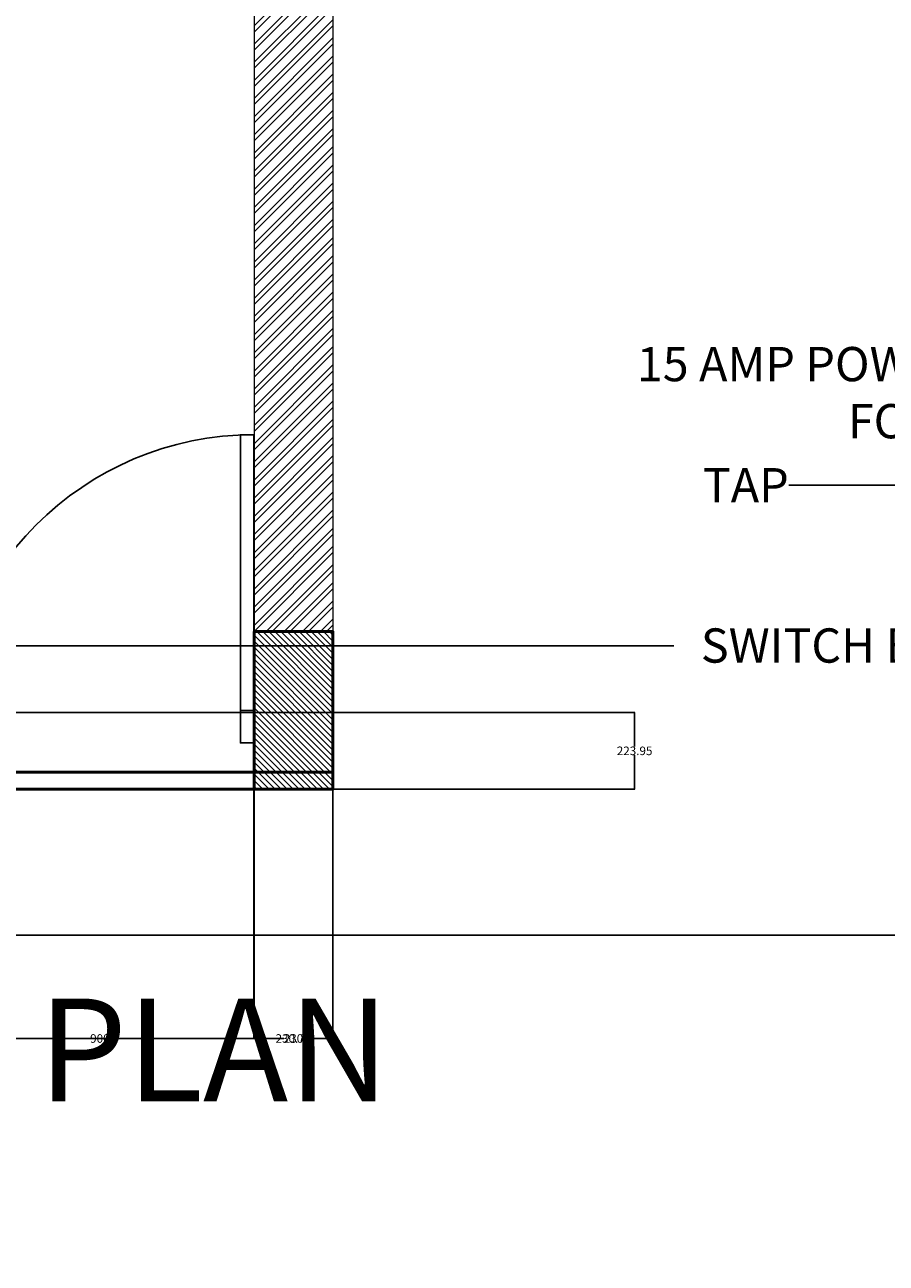
# Model space of a CAD drawing. Units: millimetres. Extents: x 1944 to 29915, y -10550 to 5909.
# Tile 6 of 24: x 9226 to 11743, y -1353 to 2263. Entities that reach past the tile are written whole.
import ezdxf
from ezdxf import colors
from ezdxf.entities.mleader import LeaderData, LeaderLine
from ezdxf.math import Vec2, Vec3

# ---------------------------------------------------------------- set-up
doc = ezdxf.new("R2010")
doc.units = ezdxf.units.MM
doc.header["$MEASUREMENT"] = 0
for name, color, linetype, lineweight in [('A-ANNO-DIMS', 2, 'Continuous', 18), ('A-ANNO-TEXT', 7, 'Continuous', 25), ('A-DOOR', 4, 'Continuous', 25), ('A-FLOR-FIXT', 9, 'Continuous', 18), ('A-WALL', 7, 'Continuous', 50), ('A-WALL-PATT', 8, 'Continuous', 18)]:
    doc.layers.add(name, color=color, linetype=linetype, lineweight=lineweight)
doc.styles.get("Standard").update_dxf_attribs({"font": 'arial.ttf'})
doc.dimstyles.get("Standard").update_dxf_attribs({"dimtxt": 25, "dimasz": 0.18, "dimexe": 0.18, "dimexo": 0.0625, "dimgap": 0.09, "dimtad": 0, "dimtih": 1, "dimtoh": 1, "dimdec": 0, "dimzin": 0, "dimdsep": 46, "dimtxsty": 'Standard', "dimcen": 0.09, "dimadec": 0, "dimazin": 0, "dimtfac": 1, "dimtdec": 0, "dimtofl": 0, "dimtmove": 0, "dimatfit": 3, "dimfxl": 1, "dimtolj": 1, "dimtzin": 0, "dimarcsym": 0})

# ---------------------------------------------------------------- blocks, each defined once
blk = doc.blocks.new('*U2')
for p, q in [((0, 0), (0, -6)), ((40, 0), (40, -6))]:
    blk.add_line(p, q)
blk.add_lwpolyline([(0, 0), (0, 40), (1.75, 40), (1.75, 0)], close=True)
blk.add_arc((0, 0), 40, 0, 90)
blk = doc.blocks.new('*D50')
at = {"layer": 'A-ANNO-DIMS', "color": 0, "lineweight": -2, "transparency": 16777216}
for p, q in [((8995.2, 30.8), (8995.2, -697.2)), ((9895.2, 30.8), (9895.2, -697.2)), ((8995.4, -697), (9417.6, -697)), ((9895, -697), (9472.9, -697))]:
    blk.add_line(p, q, dxfattribs=at)
at = {"layer": 'A-ANNO-DIMS', "color": 0, "transparency": 16777216}
for points in [[(8995.4, -697), (8995.4, -697.1), (8995.2, -697)], [(9895, -697), (9895, -697.1), (9895.2, -697)]]:
    blk.add_solid(points, dxfattribs=at)
at = {"layer": 'Defpoints', "color": 0, "transparency": 16777216}
for p in [(8995.2, 30.8), (9895.2, 30.8), (9895.2, -697)]:
    blk.add_point(p, dxfattribs=at)
at = {"layer": 'A-ANNO-DIMS', "color": 0, "transparency": 16777216, "insert": (9445.2, -697), "char_height": 25, "attachment_point": 5}
blk.add_mtext('\\A1;900', dxfattribs=at)
blk = doc.blocks.new('*D51')
at = {"layer": 'A-ANNO-DIMS', "color": 0, "lineweight": -2, "transparency": 16777216}
for p, q in [((9895.2, 30.8), (9895.2, -697.2)), ((10125.9, 30.8), (10125.9, -697.2)), ((9895.4, -697), (9958.4, -697)), ((10125.8, -697), (10062.8, -697))]:
    blk.add_line(p, q, dxfattribs=at)
at = {"layer": 'A-ANNO-DIMS', "color": 0, "transparency": 16777216}
for points in [[(9895.4, -697), (9895.4, -697.1), (9895.2, -697)], [(10125.8, -697), (10125.8, -697.1), (10125.9, -697)]]:
    blk.add_solid(points, dxfattribs=at)
at = {"layer": 'Defpoints', "color": 0, "transparency": 16777216}
for p in [(9895.2, 30.8), (10125.9, 30.8), (10125.9, -697)]:
    blk.add_point(p, dxfattribs=at)
at = {"layer": 'A-ANNO-DIMS', "color": 0, "transparency": 16777216, "insert": (10010.6, -697), "char_height": 25, "attachment_point": 5}
blk.add_mtext('\\A1;230.73', dxfattribs=at)
blk = doc.blocks.new('*D53')
at = {"layer": 'A-ANNO-DIMS', "color": 0, "lineweight": -2, "transparency": 16777216}
for p, q in [((6945.94205, 490.774608), (6945.94205, -697.212556)), ((9895.94205, 490.774608), (9895.94205, -697.212556)), ((6946.12205, -697.032556), (8383.35205, -697.032556)), ((9895.76205, -697.032556), (8458.53205, -697.032556))]:
    blk.add_line(p, q, dxfattribs=at)
at = {"layer": 'A-ANNO-DIMS', "color": 0, "transparency": 16777216}
for points in [[(6946.12205, -697.002556), (6946.12205, -697.062556), (6945.94205, -697.032556)], [(9895.76205, -697.002556), (9895.76205, -697.062556), (9895.94205, -697.032556)]]:
    blk.add_solid(points, dxfattribs=at)
at = {"layer": 'Defpoints', "color": 0, "transparency": 16777216}
for p in [(6945.94205, 490.837108), (9895.94205, 490.837108), (9895.94205, -697.032556)]:
    blk.add_point(p, dxfattribs=at)
at = {"layer": 'A-ANNO-DIMS', "color": 0, "transparency": 16777216, "insert": (8420.94205, -697.032556), "char_height": 25, "attachment_point": 5}
blk.add_mtext('\\A1;2950', dxfattribs=at)
blk = doc.blocks.new('*D54')
at = {"layer": 'A-ANNO-DIMS', "color": 0, "lineweight": -2, "transparency": 16777216}
for p, q in [((9895.9, 490.8), (9895.9, -697.2)), ((10125.9, 490.8), (10125.9, -697.2)), ((9896.1, -697), (9983.1, -697)), ((10125.8, -697), (10038.8, -697))]:
    blk.add_line(p, q, dxfattribs=at)
at = {"layer": 'A-ANNO-DIMS', "color": 0, "transparency": 16777216}
for points in [[(9896.1, -697), (9896.1, -697.1), (9895.9, -697)], [(10125.8, -697), (10125.8, -697.1), (10125.9, -697)]]:
    blk.add_solid(points, dxfattribs=at)
at = {"layer": 'Defpoints', "color": 0, "transparency": 16777216}
for p in [(9895.9, 490.8), (10125.9, 490.8), (10125.9, -697)]:
    blk.add_point(p, dxfattribs=at)
at = {"layer": 'A-ANNO-DIMS', "color": 0, "transparency": 16777216, "insert": (10010.9, -697), "char_height": 25, "attachment_point": 5}
blk.add_mtext('\\A1;230', dxfattribs=at)
blk = doc.blocks.new('*D56')
at = {"layer": 'A-ANNO-DIMS', "color": 0, "lineweight": -2, "transparency": 16777216}
for p, q in [((8999.7, 254.8), (11007.7, 254.8)), ((11007.5, 254.6), (11007.5, 155.7)), ((11007.5, 31), (11007.5, 130)), ((8995.3, 30.8), (11007.7, 30.8))]:
    blk.add_line(p, q, dxfattribs=at)
at = {"layer": 'A-ANNO-DIMS', "color": 0, "transparency": 16777216}
for points in [[(11007.5, 254.6), (11007.5, 254.6), (11007.5, 254.8)], [(11007.5, 31), (11007.5, 31), (11007.5, 30.8)]]:
    blk.add_solid(points, dxfattribs=at)
at = {"layer": 'Defpoints', "color": 0, "transparency": 16777216}
for p in [(8999.6, 254.8), (8995.2, 30.8), (11007.5, 30.8)]:
    blk.add_point(p, dxfattribs=at)
at = {"layer": 'A-ANNO-DIMS', "color": 0, "transparency": 16777216, "insert": (11007.5, 142.8), "char_height": 25, "attachment_point": 5}
blk.add_mtext('\\A1;223.95', dxfattribs=at)
blk = doc.blocks.new('*D85')
at = {"layer": 'A-ANNO-DIMS', "color": 0, "lineweight": -2, "transparency": 16777216}
for p, q in [((6418.3, -1730.7), (6418.3, -395.6)), ((6418.5, -395.8), (15860.3, -395.8)), ((25389.1, -395.8), (15947.3, -395.8)), ((25389.3, -1846.5), (25389.3, -395.6))]:
    blk.add_line(p, q, dxfattribs=at)
at = {"layer": 'A-ANNO-DIMS', "color": 0, "transparency": 16777216}
for points in [[(6418.5, -395.7), (6418.5, -395.8), (6418.3, -395.8)], [(25389.1, -395.7), (25389.1, -395.8), (25389.3, -395.8)]]:
    blk.add_solid(points, dxfattribs=at)
at = {"layer": 'Defpoints', "color": 0, "transparency": 16777216}
for p in [(25389.3, -395.8), (6418.3, -1730.8), (25389.3, -1846.5)]:
    blk.add_point(p, dxfattribs=at)
at = {"layer": 'A-ANNO-DIMS', "color": 0, "transparency": 16777216, "insert": (15903.8, -395.8), "char_height": 25, "attachment_point": 5}
blk.add_mtext('\\A1;18971', dxfattribs=at)

msp = doc.modelspace()

# ---------------------------------------------------------------- hatches: boundary and pattern name
at = {"layer": 'A-WALL-PATT'}
h = msp.add_hatch(dxfattribs=at)
h.set_pattern_fill('ANSI32', color=256, scale=100)
h.paths.add_polyline_path([(9895.942, 490.837), (10125.942, 490.837), (10125.942, 4760.837), (9895.942, 4760.837)])
h = msp.add_hatch(dxfattribs=at)
h.set_pattern_fill('ANSI31', color=256, scale=100, angle=90)
h.paths.add_polyline_path([(9895.942, 30.837), (10125.942, 30.837), (10125.942, 490.837), (9895.942, 490.837)])

# ---------------------------------------------------------------- linework, layer by layer
at = {"layer": 'A-DOOR'}
msp.add_line((9855.842, 260.837), (9895.942, 260.837), dxfattribs=at)
at = {"layer": 'A-FLOR-FIXT'}
for points in [[(9895.942, 4990.837), (10125.942, 4990.837), (10125.942, 30.837), (9895.217, 30.837)], [(9895.942, 4760.837), (9895.942, 260.837), (9855.842, 260.837)]]:
    msp.add_lwpolyline(points, dxfattribs=at)
at = {"layer": 'A-WALL'}
for p, q in [((10125.942, 81.017), (6715.942, 81.017)), ((10125.942, 30.837), (6715.942, 30.837)), ((8995.217, 30.837), (9895.942, 30.837))]:
    msp.add_line(p, q, dxfattribs=at)
msp.add_lwpolyline([(9895.942, 490.837), (10125.942, 490.837), (10125.942, 30.837), (9895.942, 30.837)], close=True, dxfattribs=at)

# ---------------------------------------------------------------- block references
at = {"layer": 'A-DOOR', "xscale": -22.5, "yscale": 22.5, "zscale": 22.5}
msp.add_blockref('*U2', (9895.217, 165.837), dxfattribs=at)

# ---------------------------------------------------------------- texts
at = {"layer": 'A-ANNO-TEXT'}
msp.add_text('KITCHEN PLAN ', height=300, dxfattribs=at).set_placement((7448.016, -880.236))

# ---------------------------------------------------------------- dimensions: what is measured, and where the dimension line sits
at = {"layer": 'A-ANNO-DIMS'}
for base, p1, p2, override, picture, middle in [((9895.942, -697.033), (6945.942, 490.837), (9895.942, 490.837), {"dimdec": 0, "dimlfac": 1, "dimrnd": 0, "dimzin": 0, "dimdsep": 46, "dimlunit": 2}, '*D53', (8420.942, -697.033)), ((10125.942, -697.033), (9895.942, 490.837), (10125.942, 490.837), {"dimdec": 0, "dimlfac": 1, "dimrnd": 0, "dimzin": 0, "dimdsep": 46, "dimlunit": 2}, '*D54', (10010.942, -697.033)), ((9895.217, -697.033), (8995.217, 30.837), (9895.217, 30.837), {"dimdec": 0, "dimlfac": 1, "dimrnd": 0, "dimzin": 0, "dimdsep": 46, "dimlunit": 2}, '*D50', (9445.217, -697.033)), ((10125.94205, -697.03256), (9895.217, 30.83711), (10125.94205, 30.83711), {"dimdec": 2, "dimlfac": 1, "dimrnd": 0, "dimzin": 0, "dimdsep": 46, "dimlunit": 2}, '*D51', (10010.57953, -697.03256)), ((25389.297, -395.752), (6418.315, -1730.752), (25389.297, -1846.542), {"dimdec": 0, "dimlfac": 1, "dimrnd": 0, "dimzin": 0, "dimdsep": 46, "dimlunit": 2}, '*D85', (15903.806, -395.752))]:
    dim = msp.add_linear_dim(base=base, p1=p1, p2=p2, dimstyle='Standard', override=override, dxfattribs=at)
    dim.commit()
    dim.dimension.update_dxf_attribs({"geometry": picture, "text_midpoint": middle})
dim = msp.add_linear_dim(base=(11007.504, 30.837), p1=(8999.621, 254.791), p2=(8995.217, 30.837), angle=90, dimstyle='Standard', override={"dimdec": 2, "dimlfac": 1, "dimrnd": 0, "dimzin": 0, "dimdsep": 46, "dimlunit": 2}, dxfattribs=at)
dim.commit()
dim.dimension.update_dxf_attribs({"geometry": '*D56', "text_midpoint": (11007.504, 142.814)})

# ---------------------------------------------------------------- leaders
at = {"layer": 'A-ANNO-TEXT'}
ml = msp.add_multileader_mtext('Standard', dxfattribs=at)
ml.set_content('15 AMP POWER POINT \\PFOR GEYSER ', color=256)
ml.set_leader_properties()
ml.build(insert=Vec2(0, 0))
ml.multileader.update_dxf_attribs({"dogleg_length": 0.36, "arrow_head_size": 100})
ctx = ml.context
ctx.base_point, ctx.char_height, ctx.arrow_head_size, ctx.landing_gap_size, ctx.plane_origin = Vec3(10908.052, 1271.067), 100, 100, 0.09, Vec3(12988.354, 1271.067)
ctx.text_align_type = 2
notes = []
notes.append((ctx, [(0, (1, 1, 0), (12988.354, 1271.067), (-1, 0), 568.936, [(0, [(14591.122, 1267.898)], 0, [])])]))
ctx.mtext.insert, ctx.mtext.alignment, ctx.mtext.flow_direction = Vec3(12419.329, 1321.919), 3, 5
ml = msp.add_multileader_mtext('Standard', dxfattribs=at)
ml.set_content('TAP', color=256)
ml.set_leader_properties()
ml.build(insert=Vec2(0, 0))
ml.multileader.update_dxf_attribs({"dogleg_length": 568.936, "arrow_head_size": 100})
ctx = ml.context
ctx.base_point, ctx.char_height, ctx.arrow_head_size, ctx.landing_gap_size, ctx.plane_origin = Vec3(11195.309, 918.379), 100, 100, 0.09, Vec3(12026.771, 918.379)
ctx.text_align_type = 2
notes.append((ctx, [(0, (1, 1, 0), (12026.771, 918.379), (-1, 0), 568.936, [(0, [(13257.147, 1072.171)], 0, [])])]))
ctx.mtext.insert, ctx.mtext.alignment, ctx.mtext.flow_direction = Vec3(11457.746, 968.379), 3, 5
ml = msp.add_multileader_mtext('Standard', dxfattribs=at)
ml.set_content('SWITCH BOARD', color=256)
ml.set_leader_properties()
ml.build(insert=Vec2(0, 0))
ml.multileader.update_dxf_attribs({"dogleg_length": 568.936, "arrow_head_size": 100})
ctx = ml.context
ctx.base_point, ctx.char_height, ctx.arrow_head_size, ctx.landing_gap_size, ctx.plane_origin = Vec3(11122.176, 449.474), 100, 100, 0.09, Vec3(10553.24, 449.474)
ctx.text_align_type = 2
notes.append((ctx, [(0, (1, 1, 0), (10553.24, 449.474), (1, 0), 568.936, [(0, [(8914.665, 260.837), (8914.665, 449.474)], 0, [])])]))
ctx.mtext.insert, ctx.mtext.alignment, ctx.mtext.flow_direction = Vec3(12195.117, 500.327), 3, 5
for ctx, leaders in notes:
    for number, flags, end, landing, length, lines in leaders:
        leader = LeaderData()
        leader.index, (leader.has_last_leader_line, leader.has_dogleg_vector, leader.attachment_direction) = number, flags
        leader.last_leader_point, leader.dogleg_vector, leader.dogleg_length = Vec3(end), Vec3(landing), length
        for number, points, colour, breaks in lines:
            line = LeaderLine()
            line.index, line.vertices, line.color, line.breaks = number, Vec3.list(points), colors.encode_raw_color(colour), breaks
            leader.lines.append(line)
        ctx.leaders.append(leader)

doc.saveas('drawing.dxf')
